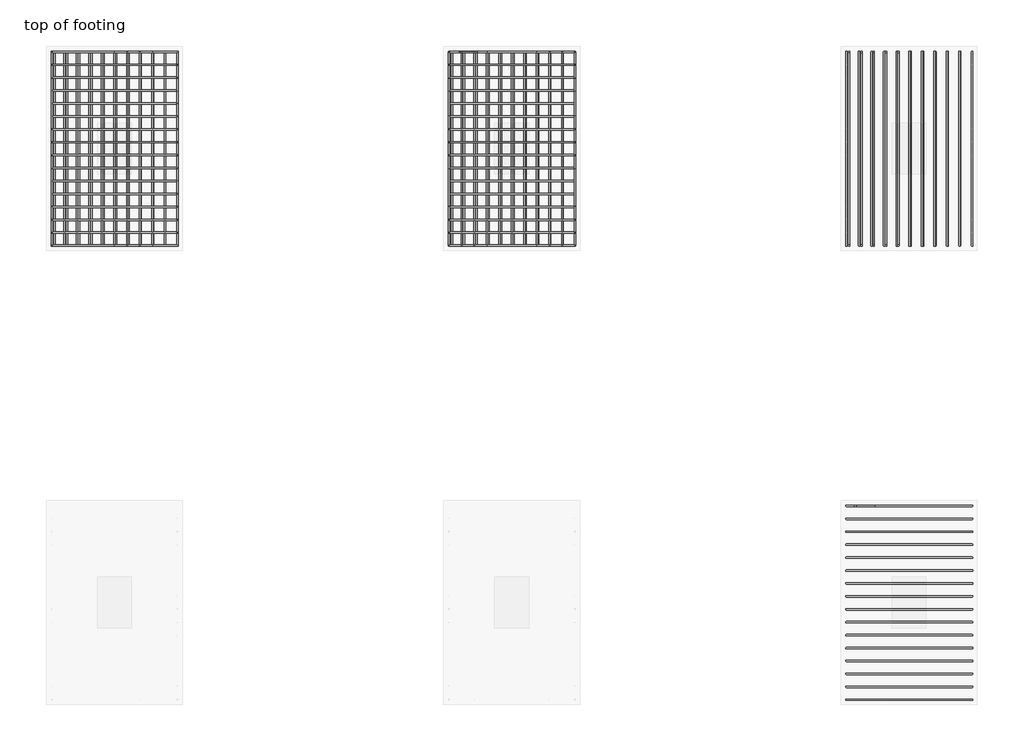
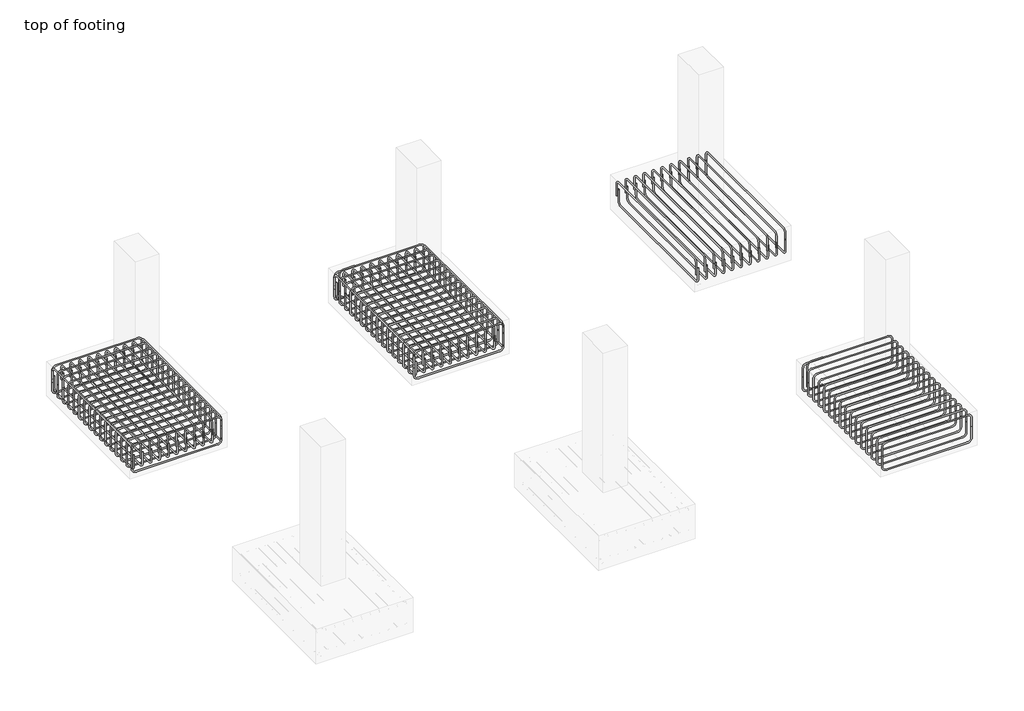
# One storey, part 5 of 8: 14 reinforcing bars.
"""IFC4 building model written with IfcOpenShell, lengths in millimetres."""

from ifc_helpers import new_model, si_unit, point, frame, origin, place, context, project, spatial, polyline, circle_curve, trimmed, segment, composite_curve, source, transform, mapped, element, save
from ifc_brep_helpers import swept_disk

model = new_model("IFC4")

# Units and contexts
model_context = context("Model", 3, world=origin())
ifc_project = project(units=[si_unit("LENGTHUNIT", "METRE", prefix="MILLI")], contexts=[model_context])

# Site, building, storey
site = spatial("IfcSite", under=ifc_project)
building = spatial("IfcBuilding", under=site)
storey = spatial("IfcBuildingStorey", under=building, Name="top of footing", Elevation=-1828.8)

# Reinforcing bars
placement = place(None, origin())
reinforcing_bar_shape = source(origin(), model_context, "Body", "SolidModel", [
    swept_disk(composite_curve([segment(polyline([(-7185.4300189, 12682.8075251, -2014.4920065), (-7185.4300189, 12682.8075251, -2161.7920065)]), True, "CONTINUOUS"), segment(trimmed(circle_curve(frame((-7185.4300189, 12729.1575251, -2161.7920065), z_axis=(1.0, 0.0, 0.0), x_axis=(0.0, -46.350000000000364, 0.0)), 46.35), [point((-7185.4300189, 12682.8075251, -2161.7920065))], [point((-7185.4300189, 12729.1575251, -2208.1420065))], True, "CARTESIAN"), True, "CONTINUOUS"), segment(polyline([(-7185.4300189, 12729.1575251, -2208.1420065), (-7185.4300189, 14343.7575251, -2208.1420065)]), True, "CONTINUOUS"), segment(trimmed(circle_curve(frame((-7185.4300189, 14343.7575251, -2161.7920065), z_axis=(1.0, 0.0, 0.0), x_axis=(0.0, 0.0, -46.350000000000364)), 46.35), [point((-7185.4300189, 14343.7575251, -2208.1420065))], [point((-7185.4300189, 14390.1075251, -2161.7920065))], True, "CARTESIAN"), True, "CONTINUOUS"), segment(polyline([(-7185.4300189, 14390.1075251, -2161.7920065), (-7185.4300189, 14390.1075251, -2014.4920065)]), True, "CONTINUOUS")], self_intersect=False), 6.35),
])
element("IfcReinforcingBar", 1, at=placement, inside=storey, context=model_context, shape_type="MappedRepresentation", body=[
    mapped(reinforcing_bar_shape, transform((0.0, 0.0, 0.0), x_axis=(1.0, 0.0, 0.0), y_axis=(0.0, 1.0, 0.0), z_axis=(0.0, 0.0, 1.0))),
    mapped(reinforcing_bar_shape, transform((-108.3645139, 0.0, 0.0), x_axis=(1.0, 0.0, 0.0), y_axis=(0.0, 1.0, 0.0), z_axis=(0.0, 0.0, 1.0))),
    mapped(reinforcing_bar_shape, transform((-216.7290279, 0.0, 0.0), x_axis=(1.0, 0.0, 0.0), y_axis=(0.0, 1.0, 0.0), z_axis=(0.0, 0.0, 1.0))),
    mapped(reinforcing_bar_shape, transform((-325.0935418, 0.0, 0.0), x_axis=(1.0, 0.0, 0.0), y_axis=(0.0, 1.0, 0.0), z_axis=(0.0, 0.0, 1.0))),
    mapped(reinforcing_bar_shape, transform((-433.4580557, 0.0, 0.0), x_axis=(1.0, 0.0, 0.0), y_axis=(0.0, 1.0, 0.0), z_axis=(0.0, 0.0, 1.0))),
    mapped(reinforcing_bar_shape, transform((-541.8225696, 0.0, 0.0), x_axis=(1.0, 0.0, 0.0), y_axis=(0.0, 1.0, 0.0), z_axis=(0.0, 0.0, 1.0))),
    mapped(reinforcing_bar_shape, transform((-650.1870836, 0.0, 0.0), x_axis=(1.0, 0.0, 0.0), y_axis=(0.0, 1.0, 0.0), z_axis=(0.0, 0.0, 1.0))),
    mapped(reinforcing_bar_shape, transform((-758.5515975, 0.0, 0.0), x_axis=(1.0, 0.0, 0.0), y_axis=(0.0, 1.0, 0.0), z_axis=(0.0, 0.0, 1.0))),
    mapped(reinforcing_bar_shape, transform((-866.9161114, 0.0, 0.0), x_axis=(1.0, 0.0, 0.0), y_axis=(0.0, 1.0, 0.0), z_axis=(0.0, 0.0, 1.0))),
    mapped(reinforcing_bar_shape, transform((-975.2806253, 0.0, 0.0), x_axis=(1.0, 0.0, 0.0), y_axis=(0.0, 1.0, 0.0), z_axis=(0.0, 0.0, 1.0))),
    mapped(reinforcing_bar_shape, transform((-1083.6451393, 0.0, 0.0), x_axis=(1.0, 0.0, 0.0), y_axis=(0.0, 1.0, 0.0), z_axis=(0.0, 0.0, 1.0))),
])
reinforcing_bar_2_shape = source(origin(), model_context, "Body", "SolidModel", [
    swept_disk(composite_curve([segment(polyline([(-8292.7300189, 12682.8075251, -2085.8010212), (-8292.7300189, 12682.8075251, -1938.5010212)]), True, "CONTINUOUS"), segment(trimmed(circle_curve(frame((-8292.7300189, 12729.1575251, -1938.5010212), z_axis=(-1.0, 0.0, 0.0), x_axis=(0.0, -46.350000000000364, 0.0)), 46.35), [point((-8292.7300189, 12682.8075251, -1938.5010212))], [point((-8292.7300189, 12729.1575251, -1892.1510212))], True, "CARTESIAN"), True, "CONTINUOUS"), segment(polyline([(-8292.7300189, 12729.1575251, -1892.1510212), (-8292.7300189, 14343.7575251, -1892.1510212)]), True, "CONTINUOUS"), segment(trimmed(circle_curve(frame((-8292.7300189, 14343.7575251, -1938.5010212), z_axis=(-1.0, 0.0, 0.0), x_axis=(0.0, 0.0, 46.34999999999991)), 46.35), [point((-8292.7300189, 14343.7575251, -1892.1510212))], [point((-8292.7300189, 14390.1075251, -1938.5010212))], True, "CARTESIAN"), True, "CONTINUOUS"), segment(polyline([(-8292.7300189, 14390.1075251, -1938.5010212), (-8292.7300189, 14390.1075251, -2085.8010212)]), True, "CONTINUOUS")], self_intersect=False), 6.35),
])
element("IfcReinforcingBar", 2, at=placement, inside=storey, context=model_context, shape_type="MappedRepresentation", body=[
    mapped(reinforcing_bar_2_shape, transform((0.0, 0.0, 0.0), x_axis=(1.0, 0.0, 0.0), y_axis=(0.0, 1.0, 0.0), z_axis=(0.0, 0.0, 1.0))),
    mapped(reinforcing_bar_2_shape, transform((110.73, 0.0, 0.0), x_axis=(1.0, 0.0, 0.0), y_axis=(0.0, 1.0, 0.0), z_axis=(0.0, 0.0, 1.0))),
    mapped(reinforcing_bar_2_shape, transform((221.46, 0.0, 0.0), x_axis=(1.0, 0.0, 0.0), y_axis=(0.0, 1.0, 0.0), z_axis=(0.0, 0.0, 1.0))),
    mapped(reinforcing_bar_2_shape, transform((332.19, 0.0, 0.0), x_axis=(1.0, 0.0, 0.0), y_axis=(0.0, 1.0, 0.0), z_axis=(0.0, 0.0, 1.0))),
    mapped(reinforcing_bar_2_shape, transform((442.92, 0.0, 0.0), x_axis=(1.0, 0.0, 0.0), y_axis=(0.0, 1.0, 0.0), z_axis=(0.0, 0.0, 1.0))),
    mapped(reinforcing_bar_2_shape, transform((553.65, 0.0, 0.0), x_axis=(1.0, 0.0, 0.0), y_axis=(0.0, 1.0, 0.0), z_axis=(0.0, 0.0, 1.0))),
    mapped(reinforcing_bar_2_shape, transform((664.38, 0.0, 0.0), x_axis=(1.0, 0.0, 0.0), y_axis=(0.0, 1.0, 0.0), z_axis=(0.0, 0.0, 1.0))),
    mapped(reinforcing_bar_2_shape, transform((775.11, 0.0, 0.0), x_axis=(1.0, 0.0, 0.0), y_axis=(0.0, 1.0, 0.0), z_axis=(0.0, 0.0, 1.0))),
    mapped(reinforcing_bar_2_shape, transform((885.84, 0.0, 0.0), x_axis=(1.0, 0.0, 0.0), y_axis=(0.0, 1.0, 0.0), z_axis=(0.0, 0.0, 1.0))),
    mapped(reinforcing_bar_2_shape, transform((996.57, 0.0, 0.0), x_axis=(1.0, 0.0, 0.0), y_axis=(0.0, 1.0, 0.0), z_axis=(0.0, 0.0, 1.0))),
    mapped(reinforcing_bar_2_shape, transform((1107.3, 0.0, 0.0), x_axis=(1.0, 0.0, 0.0), y_axis=(0.0, 1.0, 0.0), z_axis=(0.0, 0.0, 1.0))),
])
reinforcing_bar_3_shape = source(origin(), model_context, "Body", "SolidModel", [
    swept_disk(composite_curve([segment(polyline([(-7185.4300189, 14390.1075251, -2044.8290141), (-7185.4300189, 14390.1075251, -2192.1290141)]), True, "CONTINUOUS"), segment(trimmed(circle_curve(frame((-7231.7800189, 14390.1075251, -2192.1290141), z_axis=(0.0, 1.0, 0.0), x_axis=(46.350000000000364, 0.0, 0.0)), 46.35), [point((-7185.4300189, 14390.1075251, -2192.1290141))], [point((-7231.7800189, 14390.1075251, -2238.4790141))], True, "CARTESIAN"), True, "CONTINUOUS"), segment(polyline([(-7231.7800189, 14390.1075251, -2238.4790141), (-8246.3800189, 14390.1075251, -2238.4790141)]), True, "CONTINUOUS"), segment(trimmed(circle_curve(frame((-8246.3800189, 14390.1075251, -2192.1290141), z_axis=(0.0, 1.0, 0.0), x_axis=(0.0, 0.0, -46.34999999999991)), 46.35), [point((-8246.3800189, 14390.1075251, -2238.4790141))], [point((-8292.7300189, 14390.1075251, -2192.1290141))], True, "CARTESIAN"), True, "CONTINUOUS"), segment(polyline([(-8292.7300189, 14390.1075251, -2192.1290141), (-8292.7300189, 14390.1075251, -2044.8290141)]), True, "CONTINUOUS")], self_intersect=False), 6.35),
])
element("IfcReinforcingBar", 3, at=placement, inside=storey, context=model_context, shape_type="MappedRepresentation", body=[
    mapped(reinforcing_bar_3_shape, transform((0.0, 0.0, 0.0), x_axis=(1.0, 0.0, 0.0), y_axis=(0.0, 1.0, 0.0), z_axis=(0.0, 0.0, 1.0))),
    mapped(reinforcing_bar_3_shape, transform((0.0, -113.82, 0.0), x_axis=(1.0, 0.0, 0.0), y_axis=(0.0, 1.0, 0.0), z_axis=(0.0, 0.0, 1.0))),
    mapped(reinforcing_bar_3_shape, transform((0.0, -227.64, 0.0), x_axis=(1.0, 0.0, 0.0), y_axis=(0.0, 1.0, 0.0), z_axis=(0.0, 0.0, 1.0))),
    mapped(reinforcing_bar_3_shape, transform((0.0, -341.46, 0.0), x_axis=(1.0, 0.0, 0.0), y_axis=(0.0, 1.0, 0.0), z_axis=(0.0, 0.0, 1.0))),
    mapped(reinforcing_bar_3_shape, transform((0.0, -455.28, 0.0), x_axis=(1.0, 0.0, 0.0), y_axis=(0.0, 1.0, 0.0), z_axis=(0.0, 0.0, 1.0))),
    mapped(reinforcing_bar_3_shape, transform((0.0, -569.1, 0.0), x_axis=(1.0, 0.0, 0.0), y_axis=(0.0, 1.0, 0.0), z_axis=(0.0, 0.0, 1.0))),
    mapped(reinforcing_bar_3_shape, transform((0.0, -682.92, 0.0), x_axis=(1.0, 0.0, 0.0), y_axis=(0.0, 1.0, 0.0), z_axis=(0.0, 0.0, 1.0))),
    mapped(reinforcing_bar_3_shape, transform((0.0, -796.74, 0.0), x_axis=(1.0, 0.0, 0.0), y_axis=(0.0, 1.0, 0.0), z_axis=(0.0, 0.0, 1.0))),
    mapped(reinforcing_bar_3_shape, transform((0.0, -910.56, 0.0), x_axis=(1.0, 0.0, 0.0), y_axis=(0.0, 1.0, 0.0), z_axis=(0.0, 0.0, 1.0))),
    mapped(reinforcing_bar_3_shape, transform((0.0, -1024.38, 0.0), x_axis=(1.0, 0.0, 0.0), y_axis=(0.0, 1.0, 0.0), z_axis=(0.0, 0.0, 1.0))),
    mapped(reinforcing_bar_3_shape, transform((0.0, -1138.2, 0.0), x_axis=(1.0, 0.0, 0.0), y_axis=(0.0, 1.0, 0.0), z_axis=(0.0, 0.0, 1.0))),
    mapped(reinforcing_bar_3_shape, transform((0.0, -1252.02, 0.0), x_axis=(1.0, 0.0, 0.0), y_axis=(0.0, 1.0, 0.0), z_axis=(0.0, 0.0, 1.0))),
    mapped(reinforcing_bar_3_shape, transform((0.0, -1365.84, 0.0), x_axis=(1.0, 0.0, 0.0), y_axis=(0.0, 1.0, 0.0), z_axis=(0.0, 0.0, 1.0))),
    mapped(reinforcing_bar_3_shape, transform((0.0, -1479.66, 0.0), x_axis=(1.0, 0.0, 0.0), y_axis=(0.0, 1.0, 0.0), z_axis=(0.0, 0.0, 1.0))),
    mapped(reinforcing_bar_3_shape, transform((0.0, -1593.48, 0.0), x_axis=(1.0, 0.0, 0.0), y_axis=(0.0, 1.0, 0.0), z_axis=(0.0, 0.0, 1.0))),
    mapped(reinforcing_bar_3_shape, transform((0.0, -1707.3, 0.0), x_axis=(1.0, 0.0, 0.0), y_axis=(0.0, 1.0, 0.0), z_axis=(0.0, 0.0, 1.0))),
])
reinforcing_bar_4_shape = source(origin(), model_context, "Body", "SolidModel", [
    swept_disk(composite_curve([segment(polyline([(-8292.7300189, 14390.1075251, -2075.0801535), (-8292.7300189, 14390.1075251, -1927.7801535)]), True, "CONTINUOUS"), segment(trimmed(circle_curve(frame((-8246.3800189, 14390.1075251, -1927.7801535), z_axis=(0.0, 1.0, 0.0), x_axis=(-46.350000000000364, 0.0, 0.0)), 46.35), [point((-8292.7300189, 14390.1075251, -1927.7801535))], [point((-8246.3800189, 14390.1075251, -1881.4301535))], True, "CARTESIAN"), True, "CONTINUOUS"), segment(polyline([(-8246.3800189, 14390.1075251, -1881.4301535), (-7231.7800189, 14390.1075251, -1881.4301535)]), True, "CONTINUOUS"), segment(trimmed(circle_curve(frame((-7231.7800189, 14390.1075251, -1927.7801535), z_axis=(0.0, 1.0, 0.0), x_axis=(0.0, 0.0, 46.350000000000136)), 46.35), [point((-7231.7800189, 14390.1075251, -1881.4301535))], [point((-7185.4300189, 14390.1075251, -1927.7801535))], True, "CARTESIAN"), True, "CONTINUOUS"), segment(polyline([(-7185.4300189, 14390.1075251, -1927.7801535), (-7185.4300189, 14390.1075251, -2075.0801535)]), True, "CONTINUOUS")], self_intersect=False), 6.35),
])
element("IfcReinforcingBar", 4, at=placement, inside=storey, context=model_context, shape_type="MappedRepresentation", body=[
    mapped(reinforcing_bar_4_shape, transform((0.0, 0.0, 0.0), x_axis=(1.0, 0.0, 0.0), y_axis=(0.0, 1.0, 0.0), z_axis=(0.0, 0.0, 1.0))),
    mapped(reinforcing_bar_4_shape, transform((0.0, -113.82, 0.0), x_axis=(1.0, 0.0, 0.0), y_axis=(0.0, 1.0, 0.0), z_axis=(0.0, 0.0, 1.0))),
    mapped(reinforcing_bar_4_shape, transform((0.0, -227.64, 0.0), x_axis=(1.0, 0.0, 0.0), y_axis=(0.0, 1.0, 0.0), z_axis=(0.0, 0.0, 1.0))),
    mapped(reinforcing_bar_4_shape, transform((0.0, -341.46, 0.0), x_axis=(1.0, 0.0, 0.0), y_axis=(0.0, 1.0, 0.0), z_axis=(0.0, 0.0, 1.0))),
    mapped(reinforcing_bar_4_shape, transform((0.0, -455.28, 0.0), x_axis=(1.0, 0.0, 0.0), y_axis=(0.0, 1.0, 0.0), z_axis=(0.0, 0.0, 1.0))),
    mapped(reinforcing_bar_4_shape, transform((0.0, -569.1, 0.0), x_axis=(1.0, 0.0, 0.0), y_axis=(0.0, 1.0, 0.0), z_axis=(0.0, 0.0, 1.0))),
    mapped(reinforcing_bar_4_shape, transform((0.0, -682.92, 0.0), x_axis=(1.0, 0.0, 0.0), y_axis=(0.0, 1.0, 0.0), z_axis=(0.0, 0.0, 1.0))),
    mapped(reinforcing_bar_4_shape, transform((0.0, -796.74, 0.0), x_axis=(1.0, 0.0, 0.0), y_axis=(0.0, 1.0, 0.0), z_axis=(0.0, 0.0, 1.0))),
    mapped(reinforcing_bar_4_shape, transform((0.0, -910.56, 0.0), x_axis=(1.0, 0.0, 0.0), y_axis=(0.0, 1.0, 0.0), z_axis=(0.0, 0.0, 1.0))),
    mapped(reinforcing_bar_4_shape, transform((0.0, -1024.38, 0.0), x_axis=(1.0, 0.0, 0.0), y_axis=(0.0, 1.0, 0.0), z_axis=(0.0, 0.0, 1.0))),
    mapped(reinforcing_bar_4_shape, transform((0.0, -1138.2, 0.0), x_axis=(1.0, 0.0, 0.0), y_axis=(0.0, 1.0, 0.0), z_axis=(0.0, 0.0, 1.0))),
    mapped(reinforcing_bar_4_shape, transform((0.0, -1252.02, 0.0), x_axis=(1.0, 0.0, 0.0), y_axis=(0.0, 1.0, 0.0), z_axis=(0.0, 0.0, 1.0))),
    mapped(reinforcing_bar_4_shape, transform((0.0, -1365.84, 0.0), x_axis=(1.0, 0.0, 0.0), y_axis=(0.0, 1.0, 0.0), z_axis=(0.0, 0.0, 1.0))),
    mapped(reinforcing_bar_4_shape, transform((0.0, -1479.66, 0.0), x_axis=(1.0, 0.0, 0.0), y_axis=(0.0, 1.0, 0.0), z_axis=(0.0, 0.0, 1.0))),
    mapped(reinforcing_bar_4_shape, transform((0.0, -1593.48, 0.0), x_axis=(1.0, 0.0, 0.0), y_axis=(0.0, 1.0, 0.0), z_axis=(0.0, 0.0, 1.0))),
    mapped(reinforcing_bar_4_shape, transform((0.0, -1707.3, 0.0), x_axis=(1.0, 0.0, 0.0), y_axis=(0.0, 1.0, 0.0), z_axis=(0.0, 0.0, 1.0))),
])
reinforcing_bar_5_shape = source(origin(), model_context, "Body", "SolidModel", [
    swept_disk(composite_curve([segment(polyline([(-3685.4300189, 12682.8075251, -2014.4920065), (-3685.4300189, 12682.8075251, -2161.7920065)]), True, "CONTINUOUS"), segment(trimmed(circle_curve(frame((-3685.4300189, 12729.1575251, -2161.7920065), z_axis=(1.0, 0.0, 0.0), x_axis=(0.0, -46.350000000000364, 0.0)), 46.35), [point((-3685.4300189, 12682.8075251, -2161.7920065))], [point((-3685.4300189, 12729.1575251, -2208.1420065))], True, "CARTESIAN"), True, "CONTINUOUS"), segment(polyline([(-3685.4300189, 12729.1575251, -2208.1420065), (-3685.4300189, 14343.7575251, -2208.1420065)]), True, "CONTINUOUS"), segment(trimmed(circle_curve(frame((-3685.4300189, 14343.7575251, -2161.7920065), z_axis=(1.0, 0.0, 0.0), x_axis=(0.0, 0.0, -46.350000000000364)), 46.35), [point((-3685.4300189, 14343.7575251, -2208.1420065))], [point((-3685.4300189, 14390.1075251, -2161.7920065))], True, "CARTESIAN"), True, "CONTINUOUS"), segment(polyline([(-3685.4300189, 14390.1075251, -2161.7920065), (-3685.4300189, 14390.1075251, -2014.4920065)]), True, "CONTINUOUS")], self_intersect=False), 6.35),
])
element("IfcReinforcingBar", 5, at=placement, inside=storey, context=model_context, shape_type="MappedRepresentation", body=[
    mapped(reinforcing_bar_5_shape, transform((0.0, 0.0, 0.0), x_axis=(1.0, 0.0, 0.0), y_axis=(0.0, 1.0, 0.0), z_axis=(0.0, 0.0, 1.0))),
    mapped(reinforcing_bar_5_shape, transform((-108.3645139, 0.0, 0.0), x_axis=(1.0, 0.0, 0.0), y_axis=(0.0, 1.0, 0.0), z_axis=(0.0, 0.0, 1.0))),
    mapped(reinforcing_bar_5_shape, transform((-216.7290279, 0.0, 0.0), x_axis=(1.0, 0.0, 0.0), y_axis=(0.0, 1.0, 0.0), z_axis=(0.0, 0.0, 1.0))),
    mapped(reinforcing_bar_5_shape, transform((-325.0935418, 0.0, 0.0), x_axis=(1.0, 0.0, 0.0), y_axis=(0.0, 1.0, 0.0), z_axis=(0.0, 0.0, 1.0))),
    mapped(reinforcing_bar_5_shape, transform((-433.4580557, 0.0, 0.0), x_axis=(1.0, 0.0, 0.0), y_axis=(0.0, 1.0, 0.0), z_axis=(0.0, 0.0, 1.0))),
    mapped(reinforcing_bar_5_shape, transform((-541.8225696, 0.0, 0.0), x_axis=(1.0, 0.0, 0.0), y_axis=(0.0, 1.0, 0.0), z_axis=(0.0, 0.0, 1.0))),
    mapped(reinforcing_bar_5_shape, transform((-650.1870836, 0.0, 0.0), x_axis=(1.0, 0.0, 0.0), y_axis=(0.0, 1.0, 0.0), z_axis=(0.0, 0.0, 1.0))),
    mapped(reinforcing_bar_5_shape, transform((-758.5515975, 0.0, 0.0), x_axis=(1.0, 0.0, 0.0), y_axis=(0.0, 1.0, 0.0), z_axis=(0.0, 0.0, 1.0))),
    mapped(reinforcing_bar_5_shape, transform((-866.9161114, 0.0, 0.0), x_axis=(1.0, 0.0, 0.0), y_axis=(0.0, 1.0, 0.0), z_axis=(0.0, 0.0, 1.0))),
    mapped(reinforcing_bar_5_shape, transform((-975.2806253, 0.0, 0.0), x_axis=(1.0, 0.0, 0.0), y_axis=(0.0, 1.0, 0.0), z_axis=(0.0, 0.0, 1.0))),
    mapped(reinforcing_bar_5_shape, transform((-1083.6451393, 0.0, 0.0), x_axis=(1.0, 0.0, 0.0), y_axis=(0.0, 1.0, 0.0), z_axis=(0.0, 0.0, 1.0))),
])
reinforcing_bar_6_shape = source(origin(), model_context, "Body", "SolidModel", [
    swept_disk(composite_curve([segment(polyline([(-4792.7300189, 12682.8075251, -2085.8010212), (-4792.7300189, 12682.8075251, -1938.5010212)]), True, "CONTINUOUS"), segment(trimmed(circle_curve(frame((-4792.7300189, 12729.1575251, -1938.5010212), z_axis=(-1.0, 0.0, 0.0), x_axis=(0.0, -46.350000000000364, 0.0)), 46.35), [point((-4792.7300189, 12682.8075251, -1938.5010212))], [point((-4792.7300189, 12729.1575251, -1892.1510212))], True, "CARTESIAN"), True, "CONTINUOUS"), segment(polyline([(-4792.7300189, 12729.1575251, -1892.1510212), (-4792.7300189, 14343.7575251, -1892.1510212)]), True, "CONTINUOUS"), segment(trimmed(circle_curve(frame((-4792.7300189, 14343.7575251, -1938.5010212), z_axis=(-1.0, 0.0, 0.0), x_axis=(0.0, 0.0, 46.34999999999991)), 46.35), [point((-4792.7300189, 14343.7575251, -1892.1510212))], [point((-4792.7300189, 14390.1075251, -1938.5010212))], True, "CARTESIAN"), True, "CONTINUOUS"), segment(polyline([(-4792.7300189, 14390.1075251, -1938.5010212), (-4792.7300189, 14390.1075251, -2085.8010212)]), True, "CONTINUOUS")], self_intersect=False), 6.35),
])
element("IfcReinforcingBar", 6, at=placement, inside=storey, context=model_context, shape_type="MappedRepresentation", body=[
    mapped(reinforcing_bar_6_shape, transform((0.0, 0.0, 0.0), x_axis=(1.0, 0.0, 0.0), y_axis=(0.0, 1.0, 0.0), z_axis=(0.0, 0.0, 1.0))),
    mapped(reinforcing_bar_6_shape, transform((110.73, 0.0, 0.0), x_axis=(1.0, 0.0, 0.0), y_axis=(0.0, 1.0, 0.0), z_axis=(0.0, 0.0, 1.0))),
    mapped(reinforcing_bar_6_shape, transform((221.46, 0.0, 0.0), x_axis=(1.0, 0.0, 0.0), y_axis=(0.0, 1.0, 0.0), z_axis=(0.0, 0.0, 1.0))),
    mapped(reinforcing_bar_6_shape, transform((332.19, 0.0, 0.0), x_axis=(1.0, 0.0, 0.0), y_axis=(0.0, 1.0, 0.0), z_axis=(0.0, 0.0, 1.0))),
    mapped(reinforcing_bar_6_shape, transform((442.92, 0.0, 0.0), x_axis=(1.0, 0.0, 0.0), y_axis=(0.0, 1.0, 0.0), z_axis=(0.0, 0.0, 1.0))),
    mapped(reinforcing_bar_6_shape, transform((553.65, 0.0, 0.0), x_axis=(1.0, 0.0, 0.0), y_axis=(0.0, 1.0, 0.0), z_axis=(0.0, 0.0, 1.0))),
    mapped(reinforcing_bar_6_shape, transform((664.38, 0.0, 0.0), x_axis=(1.0, 0.0, 0.0), y_axis=(0.0, 1.0, 0.0), z_axis=(0.0, 0.0, 1.0))),
    mapped(reinforcing_bar_6_shape, transform((775.11, 0.0, 0.0), x_axis=(1.0, 0.0, 0.0), y_axis=(0.0, 1.0, 0.0), z_axis=(0.0, 0.0, 1.0))),
    mapped(reinforcing_bar_6_shape, transform((885.84, 0.0, 0.0), x_axis=(1.0, 0.0, 0.0), y_axis=(0.0, 1.0, 0.0), z_axis=(0.0, 0.0, 1.0))),
    mapped(reinforcing_bar_6_shape, transform((996.57, 0.0, 0.0), x_axis=(1.0, 0.0, 0.0), y_axis=(0.0, 1.0, 0.0), z_axis=(0.0, 0.0, 1.0))),
    mapped(reinforcing_bar_6_shape, transform((1107.3, 0.0, 0.0), x_axis=(1.0, 0.0, 0.0), y_axis=(0.0, 1.0, 0.0), z_axis=(0.0, 0.0, 1.0))),
])
element("IfcReinforcingBar", 7, at=placement, inside=storey, context=model_context, shape_type="SolidModel", body=[
    swept_disk(composite_curve([segment(polyline([(-4543.0309105, 14390.1075251, -2232.45), (-4690.3309105, 14390.1075251, -2232.45)]), True, "CONTINUOUS"), segment(trimmed(circle_curve(frame((-4690.3309105, 14390.1075251, -2186.1), z_axis=(0.0, 1.0, 0.0), x_axis=(0.0, 0.0, -46.34999999999991)), 46.35), [point((-4690.3309105, 14390.1075251, -2232.45))], [point((-4736.6809105, 14390.1075251, -2186.1))], True, "CARTESIAN"), True, "CONTINUOUS"), segment(polyline([(-4736.6809105, 14390.1075251, -2186.1), (-4736.6809105, 14390.1075251, -1921.5)]), True, "CONTINUOUS"), segment(trimmed(circle_curve(frame((-4690.3309105, 14390.1075251, -1921.5), z_axis=(0.0, 1.0, 0.0), x_axis=(-46.350000000000364, 0.0, 0.0)), 46.35), [point((-4736.6809105, 14390.1075251, -1921.5))], [point((-4690.3309105, 14390.1075251, -1875.15))], True, "CARTESIAN"), True, "CONTINUOUS"), segment(polyline([(-4690.3309105, 14390.1075251, -1875.15), (-4543.0309105, 14390.1075251, -1875.15)]), True, "CONTINUOUS")], self_intersect=False), 6.35),
])
reinforcing_bar_7_shape = source(origin(), model_context, "Body", "SolidModel", [
    swept_disk(composite_curve([segment(polyline([(-3685.4300189, 14390.1075251, -2044.8290141), (-3685.4300189, 14390.1075251, -2192.1290141)]), True, "CONTINUOUS"), segment(trimmed(circle_curve(frame((-3731.7800189, 14390.1075251, -2192.1290141), z_axis=(0.0, 1.0, 0.0), x_axis=(46.34999999999991, 0.0, 0.0)), 46.35), [point((-3685.4300189, 14390.1075251, -2192.1290141))], [point((-3731.7800189, 14390.1075251, -2238.4790141))], True, "CARTESIAN"), True, "CONTINUOUS"), segment(polyline([(-3731.7800189, 14390.1075251, -2238.4790141), (-4746.3800189, 14390.1075251, -2238.4790141)]), True, "CONTINUOUS"), segment(trimmed(circle_curve(frame((-4746.3800189, 14390.1075251, -2192.1290141), z_axis=(0.0, 1.0, 0.0), x_axis=(0.0, 0.0, -46.34999999999991)), 46.35), [point((-4746.3800189, 14390.1075251, -2238.4790141))], [point((-4792.7300189, 14390.1075251, -2192.1290141))], True, "CARTESIAN"), True, "CONTINUOUS"), segment(polyline([(-4792.7300189, 14390.1075251, -2192.1290141), (-4792.7300189, 14390.1075251, -2044.8290141)]), True, "CONTINUOUS")], self_intersect=False), 6.35),
])
element("IfcReinforcingBar", 8, at=placement, inside=storey, context=model_context, shape_type="MappedRepresentation", body=[
    mapped(reinforcing_bar_7_shape, transform((0.0, 0.0, 0.0), x_axis=(1.0, 0.0, 0.0), y_axis=(0.0, 1.0, 0.0), z_axis=(0.0, 0.0, 1.0))),
    mapped(reinforcing_bar_7_shape, transform((0.0, -113.82, 0.0), x_axis=(1.0, 0.0, 0.0), y_axis=(0.0, 1.0, 0.0), z_axis=(0.0, 0.0, 1.0))),
    mapped(reinforcing_bar_7_shape, transform((0.0, -227.64, 0.0), x_axis=(1.0, 0.0, 0.0), y_axis=(0.0, 1.0, 0.0), z_axis=(0.0, 0.0, 1.0))),
    mapped(reinforcing_bar_7_shape, transform((0.0, -341.46, 0.0), x_axis=(1.0, 0.0, 0.0), y_axis=(0.0, 1.0, 0.0), z_axis=(0.0, 0.0, 1.0))),
    mapped(reinforcing_bar_7_shape, transform((0.0, -455.28, 0.0), x_axis=(1.0, 0.0, 0.0), y_axis=(0.0, 1.0, 0.0), z_axis=(0.0, 0.0, 1.0))),
    mapped(reinforcing_bar_7_shape, transform((0.0, -569.1, 0.0), x_axis=(1.0, 0.0, 0.0), y_axis=(0.0, 1.0, 0.0), z_axis=(0.0, 0.0, 1.0))),
    mapped(reinforcing_bar_7_shape, transform((0.0, -682.92, 0.0), x_axis=(1.0, 0.0, 0.0), y_axis=(0.0, 1.0, 0.0), z_axis=(0.0, 0.0, 1.0))),
    mapped(reinforcing_bar_7_shape, transform((0.0, -796.74, 0.0), x_axis=(1.0, 0.0, 0.0), y_axis=(0.0, 1.0, 0.0), z_axis=(0.0, 0.0, 1.0))),
    mapped(reinforcing_bar_7_shape, transform((0.0, -910.56, 0.0), x_axis=(1.0, 0.0, 0.0), y_axis=(0.0, 1.0, 0.0), z_axis=(0.0, 0.0, 1.0))),
    mapped(reinforcing_bar_7_shape, transform((0.0, -1024.38, 0.0), x_axis=(1.0, 0.0, 0.0), y_axis=(0.0, 1.0, 0.0), z_axis=(0.0, 0.0, 1.0))),
    mapped(reinforcing_bar_7_shape, transform((0.0, -1138.2, 0.0), x_axis=(1.0, 0.0, 0.0), y_axis=(0.0, 1.0, 0.0), z_axis=(0.0, 0.0, 1.0))),
    mapped(reinforcing_bar_7_shape, transform((0.0, -1252.02, 0.0), x_axis=(1.0, 0.0, 0.0), y_axis=(0.0, 1.0, 0.0), z_axis=(0.0, 0.0, 1.0))),
    mapped(reinforcing_bar_7_shape, transform((0.0, -1365.84, 0.0), x_axis=(1.0, 0.0, 0.0), y_axis=(0.0, 1.0, 0.0), z_axis=(0.0, 0.0, 1.0))),
    mapped(reinforcing_bar_7_shape, transform((0.0, -1479.66, 0.0), x_axis=(1.0, 0.0, 0.0), y_axis=(0.0, 1.0, 0.0), z_axis=(0.0, 0.0, 1.0))),
    mapped(reinforcing_bar_7_shape, transform((0.0, -1593.48, 0.0), x_axis=(1.0, 0.0, 0.0), y_axis=(0.0, 1.0, 0.0), z_axis=(0.0, 0.0, 1.0))),
    mapped(reinforcing_bar_7_shape, transform((0.0, -1707.3, 0.0), x_axis=(1.0, 0.0, 0.0), y_axis=(0.0, 1.0, 0.0), z_axis=(0.0, 0.0, 1.0))),
])
reinforcing_bar_8_shape = source(origin(), model_context, "Body", "SolidModel", [
    swept_disk(composite_curve([segment(polyline([(-4792.7300189, 14390.1075251, -2075.0801535), (-4792.7300189, 14390.1075251, -1927.7801535)]), True, "CONTINUOUS"), segment(trimmed(circle_curve(frame((-4746.3800189, 14390.1075251, -1927.7801535), z_axis=(0.0, 1.0, 0.0), x_axis=(-46.349999999999454, 0.0, 0.0)), 46.35), [point((-4792.7300189, 14390.1075251, -1927.7801535))], [point((-4746.3800189, 14390.1075251, -1881.4301535))], True, "CARTESIAN"), True, "CONTINUOUS"), segment(polyline([(-4746.3800189, 14390.1075251, -1881.4301535), (-3731.7800189, 14390.1075251, -1881.4301535)]), True, "CONTINUOUS"), segment(trimmed(circle_curve(frame((-3731.7800189, 14390.1075251, -1927.7801535), z_axis=(0.0, 1.0, 0.0), x_axis=(0.0, 0.0, 46.350000000000136)), 46.35), [point((-3731.7800189, 14390.1075251, -1881.4301535))], [point((-3685.4300189, 14390.1075251, -1927.7801535))], True, "CARTESIAN"), True, "CONTINUOUS"), segment(polyline([(-3685.4300189, 14390.1075251, -1927.7801535), (-3685.4300189, 14390.1075251, -2075.0801535)]), True, "CONTINUOUS")], self_intersect=False), 6.35),
])
element("IfcReinforcingBar", 9, at=placement, inside=storey, context=model_context, shape_type="MappedRepresentation", body=[
    mapped(reinforcing_bar_8_shape, transform((0.0, 0.0, 0.0), x_axis=(1.0, 0.0, 0.0), y_axis=(0.0, 1.0, 0.0), z_axis=(0.0, 0.0, 1.0))),
    mapped(reinforcing_bar_8_shape, transform((0.0, -113.82, 0.0), x_axis=(1.0, 0.0, 0.0), y_axis=(0.0, 1.0, 0.0), z_axis=(0.0, 0.0, 1.0))),
    mapped(reinforcing_bar_8_shape, transform((0.0, -227.64, 0.0), x_axis=(1.0, 0.0, 0.0), y_axis=(0.0, 1.0, 0.0), z_axis=(0.0, 0.0, 1.0))),
    mapped(reinforcing_bar_8_shape, transform((0.0, -341.46, 0.0), x_axis=(1.0, 0.0, 0.0), y_axis=(0.0, 1.0, 0.0), z_axis=(0.0, 0.0, 1.0))),
    mapped(reinforcing_bar_8_shape, transform((0.0, -455.28, 0.0), x_axis=(1.0, 0.0, 0.0), y_axis=(0.0, 1.0, 0.0), z_axis=(0.0, 0.0, 1.0))),
    mapped(reinforcing_bar_8_shape, transform((0.0, -569.1, 0.0), x_axis=(1.0, 0.0, 0.0), y_axis=(0.0, 1.0, 0.0), z_axis=(0.0, 0.0, 1.0))),
    mapped(reinforcing_bar_8_shape, transform((0.0, -682.92, 0.0), x_axis=(1.0, 0.0, 0.0), y_axis=(0.0, 1.0, 0.0), z_axis=(0.0, 0.0, 1.0))),
    mapped(reinforcing_bar_8_shape, transform((0.0, -796.74, 0.0), x_axis=(1.0, 0.0, 0.0), y_axis=(0.0, 1.0, 0.0), z_axis=(0.0, 0.0, 1.0))),
    mapped(reinforcing_bar_8_shape, transform((0.0, -910.56, 0.0), x_axis=(1.0, 0.0, 0.0), y_axis=(0.0, 1.0, 0.0), z_axis=(0.0, 0.0, 1.0))),
    mapped(reinforcing_bar_8_shape, transform((0.0, -1024.38, 0.0), x_axis=(1.0, 0.0, 0.0), y_axis=(0.0, 1.0, 0.0), z_axis=(0.0, 0.0, 1.0))),
    mapped(reinforcing_bar_8_shape, transform((0.0, -1138.2, 0.0), x_axis=(1.0, 0.0, 0.0), y_axis=(0.0, 1.0, 0.0), z_axis=(0.0, 0.0, 1.0))),
    mapped(reinforcing_bar_8_shape, transform((0.0, -1252.02, 0.0), x_axis=(1.0, 0.0, 0.0), y_axis=(0.0, 1.0, 0.0), z_axis=(0.0, 0.0, 1.0))),
    mapped(reinforcing_bar_8_shape, transform((0.0, -1365.84, 0.0), x_axis=(1.0, 0.0, 0.0), y_axis=(0.0, 1.0, 0.0), z_axis=(0.0, 0.0, 1.0))),
    mapped(reinforcing_bar_8_shape, transform((0.0, -1479.66, 0.0), x_axis=(1.0, 0.0, 0.0), y_axis=(0.0, 1.0, 0.0), z_axis=(0.0, 0.0, 1.0))),
    mapped(reinforcing_bar_8_shape, transform((0.0, -1593.48, 0.0), x_axis=(1.0, 0.0, 0.0), y_axis=(0.0, 1.0, 0.0), z_axis=(0.0, 0.0, 1.0))),
    mapped(reinforcing_bar_8_shape, transform((0.0, -1707.3, 0.0), x_axis=(1.0, 0.0, 0.0), y_axis=(0.0, 1.0, 0.0), z_axis=(0.0, 0.0, 1.0))),
])
reinforcing_bar_9_shape = source(origin(), model_context, "Body", "SolidModel", [
    swept_disk(composite_curve([segment(polyline([(-185.4300189, 12682.8075251, -2014.4920065), (-185.4300189, 12682.8075251, -2161.7920065)]), True, "CONTINUOUS"), segment(trimmed(circle_curve(frame((-185.4300189, 12729.1575251, -2161.7920065), z_axis=(1.0, 0.0, 0.0), x_axis=(0.0, -46.350000000000364, 0.0)), 46.35), [point((-185.4300189, 12682.8075251, -2161.7920065))], [point((-185.4300189, 12729.1575251, -2208.1420065))], True, "CARTESIAN"), True, "CONTINUOUS"), segment(polyline([(-185.4300189, 12729.1575251, -2208.1420065), (-185.4300189, 14343.7575251, -2208.1420065)]), True, "CONTINUOUS"), segment(trimmed(circle_curve(frame((-185.4300189, 14343.7575251, -2161.7920065), z_axis=(1.0, 0.0, 0.0), x_axis=(0.0, 0.0, -46.350000000000364)), 46.35), [point((-185.4300189, 14343.7575251, -2208.1420065))], [point((-185.4300189, 14390.1075251, -2161.7920065))], True, "CARTESIAN"), True, "CONTINUOUS"), segment(polyline([(-185.4300189, 14390.1075251, -2161.7920065), (-185.4300189, 14390.1075251, -2014.4920065)]), True, "CONTINUOUS")], self_intersect=False), 6.35),
])
element("IfcReinforcingBar", 10, at=placement, inside=storey, context=model_context, shape_type="MappedRepresentation", body=[
    mapped(reinforcing_bar_9_shape, transform((0.0, 0.0, 0.0), x_axis=(1.0, 0.0, 0.0), y_axis=(0.0, 1.0, 0.0), z_axis=(0.0, 0.0, 1.0))),
    mapped(reinforcing_bar_9_shape, transform((-108.3645139, 0.0, 0.0), x_axis=(1.0, 0.0, 0.0), y_axis=(0.0, 1.0, 0.0), z_axis=(0.0, 0.0, 1.0))),
    mapped(reinforcing_bar_9_shape, transform((-216.7290279, 0.0, 0.0), x_axis=(1.0, 0.0, 0.0), y_axis=(0.0, 1.0, 0.0), z_axis=(0.0, 0.0, 1.0))),
    mapped(reinforcing_bar_9_shape, transform((-325.0935418, 0.0, 0.0), x_axis=(1.0, 0.0, 0.0), y_axis=(0.0, 1.0, 0.0), z_axis=(0.0, 0.0, 1.0))),
    mapped(reinforcing_bar_9_shape, transform((-433.4580557, 0.0, 0.0), x_axis=(1.0, 0.0, 0.0), y_axis=(0.0, 1.0, 0.0), z_axis=(0.0, 0.0, 1.0))),
    mapped(reinforcing_bar_9_shape, transform((-541.8225696, 0.0, 0.0), x_axis=(1.0, 0.0, 0.0), y_axis=(0.0, 1.0, 0.0), z_axis=(0.0, 0.0, 1.0))),
    mapped(reinforcing_bar_9_shape, transform((-650.1870836, 0.0, 0.0), x_axis=(1.0, 0.0, 0.0), y_axis=(0.0, 1.0, 0.0), z_axis=(0.0, 0.0, 1.0))),
    mapped(reinforcing_bar_9_shape, transform((-758.5515975, 0.0, 0.0), x_axis=(1.0, 0.0, 0.0), y_axis=(0.0, 1.0, 0.0), z_axis=(0.0, 0.0, 1.0))),
    mapped(reinforcing_bar_9_shape, transform((-866.9161114, 0.0, 0.0), x_axis=(1.0, 0.0, 0.0), y_axis=(0.0, 1.0, 0.0), z_axis=(0.0, 0.0, 1.0))),
    mapped(reinforcing_bar_9_shape, transform((-975.2806253, 0.0, 0.0), x_axis=(1.0, 0.0, 0.0), y_axis=(0.0, 1.0, 0.0), z_axis=(0.0, 0.0, 1.0))),
    mapped(reinforcing_bar_9_shape, transform((-1083.6451393, 0.0, 0.0), x_axis=(1.0, 0.0, 0.0), y_axis=(0.0, 1.0, 0.0), z_axis=(0.0, 0.0, 1.0))),
])
reinforcing_bar_10_shape = source(origin(), model_context, "Body", "SolidModel", [
    swept_disk(composite_curve([segment(polyline([(-1292.7300189, 12682.8075251, -2085.8010212), (-1292.7300189, 12682.8075251, -1938.5010212)]), True, "CONTINUOUS"), segment(trimmed(circle_curve(frame((-1292.7300189, 12729.1575251, -1938.5010212), z_axis=(-1.0, 0.0, 0.0), x_axis=(0.0, -46.350000000000364, 0.0)), 46.35), [point((-1292.7300189, 12682.8075251, -1938.5010212))], [point((-1292.7300189, 12729.1575251, -1892.1510212))], True, "CARTESIAN"), True, "CONTINUOUS"), segment(polyline([(-1292.7300189, 12729.1575251, -1892.1510212), (-1292.7300189, 14343.7575251, -1892.1510212)]), True, "CONTINUOUS"), segment(trimmed(circle_curve(frame((-1292.7300189, 14343.7575251, -1938.5010212), z_axis=(-1.0, 0.0, 0.0), x_axis=(0.0, 0.0, 46.34999999999991)), 46.35), [point((-1292.7300189, 14343.7575251, -1892.1510212))], [point((-1292.7300189, 14390.1075251, -1938.5010212))], True, "CARTESIAN"), True, "CONTINUOUS"), segment(polyline([(-1292.7300189, 14390.1075251, -1938.5010212), (-1292.7300189, 14390.1075251, -2085.8010212)]), True, "CONTINUOUS")], self_intersect=False), 6.35),
])
element("IfcReinforcingBar", 11, at=placement, inside=storey, context=model_context, shape_type="MappedRepresentation", body=[
    mapped(reinforcing_bar_10_shape, transform((0.0, 0.0, 0.0), x_axis=(1.0, 0.0, 0.0), y_axis=(0.0, 1.0, 0.0), z_axis=(0.0, 0.0, 1.0))),
    mapped(reinforcing_bar_10_shape, transform((110.73, 0.0, 0.0), x_axis=(1.0, 0.0, 0.0), y_axis=(0.0, 1.0, 0.0), z_axis=(0.0, 0.0, 1.0))),
    mapped(reinforcing_bar_10_shape, transform((221.46, 0.0, 0.0), x_axis=(1.0, 0.0, 0.0), y_axis=(0.0, 1.0, 0.0), z_axis=(0.0, 0.0, 1.0))),
    mapped(reinforcing_bar_10_shape, transform((332.19, 0.0, 0.0), x_axis=(1.0, 0.0, 0.0), y_axis=(0.0, 1.0, 0.0), z_axis=(0.0, 0.0, 1.0))),
    mapped(reinforcing_bar_10_shape, transform((442.92, 0.0, 0.0), x_axis=(1.0, 0.0, 0.0), y_axis=(0.0, 1.0, 0.0), z_axis=(0.0, 0.0, 1.0))),
    mapped(reinforcing_bar_10_shape, transform((553.65, 0.0, 0.0), x_axis=(1.0, 0.0, 0.0), y_axis=(0.0, 1.0, 0.0), z_axis=(0.0, 0.0, 1.0))),
    mapped(reinforcing_bar_10_shape, transform((664.38, 0.0, 0.0), x_axis=(1.0, 0.0, 0.0), y_axis=(0.0, 1.0, 0.0), z_axis=(0.0, 0.0, 1.0))),
    mapped(reinforcing_bar_10_shape, transform((775.11, 0.0, 0.0), x_axis=(1.0, 0.0, 0.0), y_axis=(0.0, 1.0, 0.0), z_axis=(0.0, 0.0, 1.0))),
    mapped(reinforcing_bar_10_shape, transform((885.84, 0.0, 0.0), x_axis=(1.0, 0.0, 0.0), y_axis=(0.0, 1.0, 0.0), z_axis=(0.0, 0.0, 1.0))),
    mapped(reinforcing_bar_10_shape, transform((996.57, 0.0, 0.0), x_axis=(1.0, 0.0, 0.0), y_axis=(0.0, 1.0, 0.0), z_axis=(0.0, 0.0, 1.0))),
    mapped(reinforcing_bar_10_shape, transform((1107.3, 0.0, 0.0), x_axis=(1.0, 0.0, 0.0), y_axis=(0.0, 1.0, 0.0), z_axis=(0.0, 0.0, 1.0))),
])
element("IfcReinforcingBar", 12, at=placement, inside=storey, context=model_context, shape_type="SolidModel", body=[
    swept_disk(composite_curve([segment(polyline([(-1043.0309105, 10390.1075251, -2232.45), (-1190.3309105, 10390.1075251, -2232.45)]), True, "CONTINUOUS"), segment(trimmed(circle_curve(frame((-1190.3309105, 10390.1075251, -2186.1), z_axis=(0.0, 1.0, 0.0), x_axis=(0.0, 0.0, -46.34999999999991)), 46.35), [point((-1190.3309105, 10390.1075251, -2232.45))], [point((-1236.6809105, 10390.1075251, -2186.1))], True, "CARTESIAN"), True, "CONTINUOUS"), segment(polyline([(-1236.6809105, 10390.1075251, -2186.1), (-1236.6809105, 10390.1075251, -1921.5)]), True, "CONTINUOUS"), segment(trimmed(circle_curve(frame((-1190.3309105, 10390.1075251, -1921.5), z_axis=(0.0, 1.0, 0.0), x_axis=(-46.34999999999991, 0.0, 0.0)), 46.35), [point((-1236.6809105, 10390.1075251, -1921.5))], [point((-1190.3309105, 10390.1075251, -1875.15))], True, "CARTESIAN"), True, "CONTINUOUS"), segment(polyline([(-1190.3309105, 10390.1075251, -1875.15), (-1043.0309105, 10390.1075251, -1875.15)]), True, "CONTINUOUS")], self_intersect=False), 6.35),
])
reinforcing_bar_11_shape = source(origin(), model_context, "Body", "SolidModel", [
    swept_disk(composite_curve([segment(polyline([(-185.4300189, 10390.1075251, -2044.8290141), (-185.4300189, 10390.1075251, -2192.1290141)]), True, "CONTINUOUS"), segment(trimmed(circle_curve(frame((-231.7800189, 10390.1075251, -2192.1290141), z_axis=(0.0, 1.0, 0.0), x_axis=(46.349999999999994, 0.0, 0.0)), 46.35), [point((-185.4300189, 10390.1075251, -2192.1290141))], [point((-231.7800189, 10390.1075251, -2238.4790141))], True, "CARTESIAN"), True, "CONTINUOUS"), segment(polyline([(-231.7800189, 10390.1075251, -2238.4790141), (-1246.3800189, 10390.1075251, -2238.4790141)]), True, "CONTINUOUS"), segment(trimmed(circle_curve(frame((-1246.3800189, 10390.1075251, -2192.1290141), z_axis=(0.0, 1.0, 0.0), x_axis=(0.0, 0.0, -46.34999999999991)), 46.35), [point((-1246.3800189, 10390.1075251, -2238.4790141))], [point((-1292.7300189, 10390.1075251, -2192.1290141))], True, "CARTESIAN"), True, "CONTINUOUS"), segment(polyline([(-1292.7300189, 10390.1075251, -2192.1290141), (-1292.7300189, 10390.1075251, -2044.8290141)]), True, "CONTINUOUS")], self_intersect=False), 6.35),
])
element("IfcReinforcingBar", 13, at=placement, inside=storey, context=model_context, shape_type="MappedRepresentation", body=[
    mapped(reinforcing_bar_11_shape, transform((0.0, 0.0, 0.0), x_axis=(1.0, 0.0, 0.0), y_axis=(0.0, 1.0, 0.0), z_axis=(0.0, 0.0, 1.0))),
    mapped(reinforcing_bar_11_shape, transform((0.0, -113.82, 0.0), x_axis=(1.0, 0.0, 0.0), y_axis=(0.0, 1.0, 0.0), z_axis=(0.0, 0.0, 1.0))),
    mapped(reinforcing_bar_11_shape, transform((0.0, -227.64, 0.0), x_axis=(1.0, 0.0, 0.0), y_axis=(0.0, 1.0, 0.0), z_axis=(0.0, 0.0, 1.0))),
    mapped(reinforcing_bar_11_shape, transform((0.0, -341.46, 0.0), x_axis=(1.0, 0.0, 0.0), y_axis=(0.0, 1.0, 0.0), z_axis=(0.0, 0.0, 1.0))),
    mapped(reinforcing_bar_11_shape, transform((0.0, -455.28, 0.0), x_axis=(1.0, 0.0, 0.0), y_axis=(0.0, 1.0, 0.0), z_axis=(0.0, 0.0, 1.0))),
    mapped(reinforcing_bar_11_shape, transform((0.0, -569.1, 0.0), x_axis=(1.0, 0.0, 0.0), y_axis=(0.0, 1.0, 0.0), z_axis=(0.0, 0.0, 1.0))),
    mapped(reinforcing_bar_11_shape, transform((0.0, -682.92, 0.0), x_axis=(1.0, 0.0, 0.0), y_axis=(0.0, 1.0, 0.0), z_axis=(0.0, 0.0, 1.0))),
    mapped(reinforcing_bar_11_shape, transform((0.0, -796.74, 0.0), x_axis=(1.0, 0.0, 0.0), y_axis=(0.0, 1.0, 0.0), z_axis=(0.0, 0.0, 1.0))),
    mapped(reinforcing_bar_11_shape, transform((0.0, -910.56, 0.0), x_axis=(1.0, 0.0, 0.0), y_axis=(0.0, 1.0, 0.0), z_axis=(0.0, 0.0, 1.0))),
    mapped(reinforcing_bar_11_shape, transform((0.0, -1024.38, 0.0), x_axis=(1.0, 0.0, 0.0), y_axis=(0.0, 1.0, 0.0), z_axis=(0.0, 0.0, 1.0))),
    mapped(reinforcing_bar_11_shape, transform((0.0, -1138.2, 0.0), x_axis=(1.0, 0.0, 0.0), y_axis=(0.0, 1.0, 0.0), z_axis=(0.0, 0.0, 1.0))),
    mapped(reinforcing_bar_11_shape, transform((0.0, -1252.02, 0.0), x_axis=(1.0, 0.0, 0.0), y_axis=(0.0, 1.0, 0.0), z_axis=(0.0, 0.0, 1.0))),
    mapped(reinforcing_bar_11_shape, transform((0.0, -1365.84, 0.0), x_axis=(1.0, 0.0, 0.0), y_axis=(0.0, 1.0, 0.0), z_axis=(0.0, 0.0, 1.0))),
    mapped(reinforcing_bar_11_shape, transform((0.0, -1479.66, 0.0), x_axis=(1.0, 0.0, 0.0), y_axis=(0.0, 1.0, 0.0), z_axis=(0.0, 0.0, 1.0))),
    mapped(reinforcing_bar_11_shape, transform((0.0, -1593.48, 0.0), x_axis=(1.0, 0.0, 0.0), y_axis=(0.0, 1.0, 0.0), z_axis=(0.0, 0.0, 1.0))),
    mapped(reinforcing_bar_11_shape, transform((0.0, -1707.3, 0.0), x_axis=(1.0, 0.0, 0.0), y_axis=(0.0, 1.0, 0.0), z_axis=(0.0, 0.0, 1.0))),
])
reinforcing_bar_12_shape = source(origin(), model_context, "Body", "SolidModel", [
    swept_disk(composite_curve([segment(polyline([(-1292.7300189, 10390.1075251, -2075.0801535), (-1292.7300189, 10390.1075251, -1927.7801535)]), True, "CONTINUOUS"), segment(trimmed(circle_curve(frame((-1246.3800189, 10390.1075251, -1927.7801535), z_axis=(0.0, 1.0, 0.0), x_axis=(-46.34999999999991, 0.0, 0.0)), 46.35), [point((-1292.7300189, 10390.1075251, -1927.7801535))], [point((-1246.3800189, 10390.1075251, -1881.4301535))], True, "CARTESIAN"), True, "CONTINUOUS"), segment(polyline([(-1246.3800189, 10390.1075251, -1881.4301535), (-231.7800189, 10390.1075251, -1881.4301535)]), True, "CONTINUOUS"), segment(trimmed(circle_curve(frame((-231.7800189, 10390.1075251, -1927.7801535), z_axis=(0.0, 1.0, 0.0), x_axis=(0.0, 0.0, 46.350000000000136)), 46.35), [point((-231.7800189, 10390.1075251, -1881.4301535))], [point((-185.4300189, 10390.1075251, -1927.7801535))], True, "CARTESIAN"), True, "CONTINUOUS"), segment(polyline([(-185.4300189, 10390.1075251, -1927.7801535), (-185.4300189, 10390.1075251, -2075.0801535)]), True, "CONTINUOUS")], self_intersect=False), 6.35),
])
element("IfcReinforcingBar", 14, at=placement, inside=storey, context=model_context, shape_type="MappedRepresentation", body=[
    mapped(reinforcing_bar_12_shape, transform((0.0, 0.0, 0.0), x_axis=(1.0, 0.0, 0.0), y_axis=(0.0, 1.0, 0.0), z_axis=(0.0, 0.0, 1.0))),
    mapped(reinforcing_bar_12_shape, transform((0.0, -113.82, 0.0), x_axis=(1.0, 0.0, 0.0), y_axis=(0.0, 1.0, 0.0), z_axis=(0.0, 0.0, 1.0))),
    mapped(reinforcing_bar_12_shape, transform((0.0, -227.64, 0.0), x_axis=(1.0, 0.0, 0.0), y_axis=(0.0, 1.0, 0.0), z_axis=(0.0, 0.0, 1.0))),
    mapped(reinforcing_bar_12_shape, transform((0.0, -341.46, 0.0), x_axis=(1.0, 0.0, 0.0), y_axis=(0.0, 1.0, 0.0), z_axis=(0.0, 0.0, 1.0))),
    mapped(reinforcing_bar_12_shape, transform((0.0, -455.28, 0.0), x_axis=(1.0, 0.0, 0.0), y_axis=(0.0, 1.0, 0.0), z_axis=(0.0, 0.0, 1.0))),
    mapped(reinforcing_bar_12_shape, transform((0.0, -569.1, 0.0), x_axis=(1.0, 0.0, 0.0), y_axis=(0.0, 1.0, 0.0), z_axis=(0.0, 0.0, 1.0))),
    mapped(reinforcing_bar_12_shape, transform((0.0, -682.92, 0.0), x_axis=(1.0, 0.0, 0.0), y_axis=(0.0, 1.0, 0.0), z_axis=(0.0, 0.0, 1.0))),
    mapped(reinforcing_bar_12_shape, transform((0.0, -796.74, 0.0), x_axis=(1.0, 0.0, 0.0), y_axis=(0.0, 1.0, 0.0), z_axis=(0.0, 0.0, 1.0))),
    mapped(reinforcing_bar_12_shape, transform((0.0, -910.56, 0.0), x_axis=(1.0, 0.0, 0.0), y_axis=(0.0, 1.0, 0.0), z_axis=(0.0, 0.0, 1.0))),
    mapped(reinforcing_bar_12_shape, transform((0.0, -1024.38, 0.0), x_axis=(1.0, 0.0, 0.0), y_axis=(0.0, 1.0, 0.0), z_axis=(0.0, 0.0, 1.0))),
    mapped(reinforcing_bar_12_shape, transform((0.0, -1138.2, 0.0), x_axis=(1.0, 0.0, 0.0), y_axis=(0.0, 1.0, 0.0), z_axis=(0.0, 0.0, 1.0))),
    mapped(reinforcing_bar_12_shape, transform((0.0, -1252.02, 0.0), x_axis=(1.0, 0.0, 0.0), y_axis=(0.0, 1.0, 0.0), z_axis=(0.0, 0.0, 1.0))),
    mapped(reinforcing_bar_12_shape, transform((0.0, -1365.84, 0.0), x_axis=(1.0, 0.0, 0.0), y_axis=(0.0, 1.0, 0.0), z_axis=(0.0, 0.0, 1.0))),
    mapped(reinforcing_bar_12_shape, transform((0.0, -1479.66, 0.0), x_axis=(1.0, 0.0, 0.0), y_axis=(0.0, 1.0, 0.0), z_axis=(0.0, 0.0, 1.0))),
    mapped(reinforcing_bar_12_shape, transform((0.0, -1593.48, 0.0), x_axis=(1.0, 0.0, 0.0), y_axis=(0.0, 1.0, 0.0), z_axis=(0.0, 0.0, 1.0))),
    mapped(reinforcing_bar_12_shape, transform((0.0, -1707.3, 0.0), x_axis=(1.0, 0.0, 0.0), y_axis=(0.0, 1.0, 0.0), z_axis=(0.0, 0.0, 1.0))),
])

save(model, "model.ifc")

# Revit data of these elements
# Elements 1, 2, 3, 4, 5, 6, 7, 8, 9, 10, 11, 12, 13, 14 (IfcReinforcingBar)
#   Phase Created = New Construction
